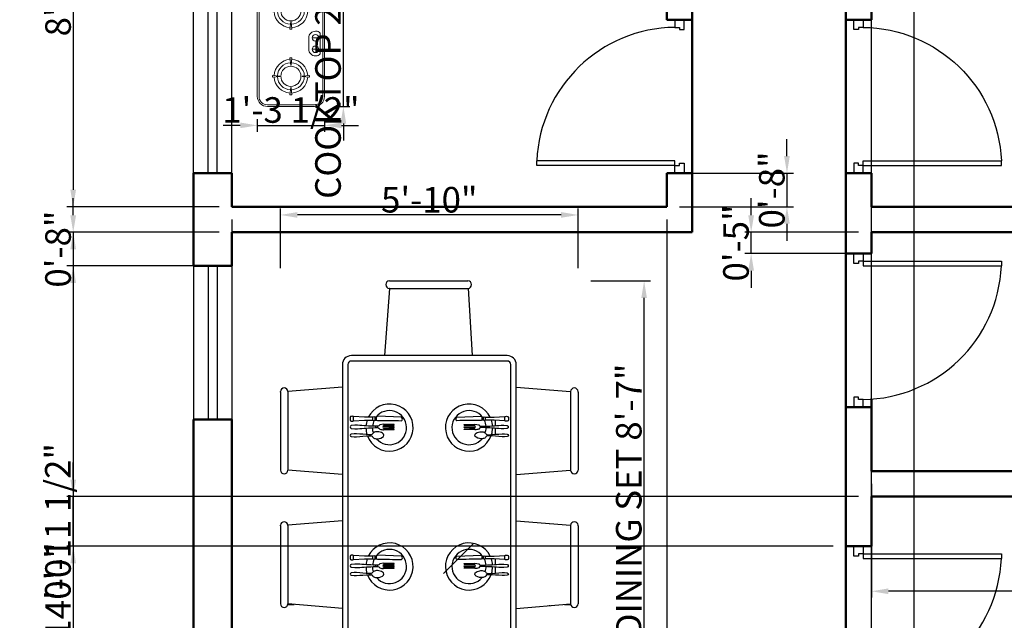
# Model space of a CAD drawing. Units: inches. Extents: x 749 to 1130, y 885 to 1490.
# Tile 3 of 5: x 749 to 980, y 1204 to 1345. Entities that reach past the tile are written whole.
import ezdxf

# ---------------------------------------------------------------- set-up
doc = ezdxf.new("R2010")
doc.units = ezdxf.units.IN
doc.header["$MEASUREMENT"] = 0
doc.layers.add('a patt', color=33, linetype='Continuous')
for name, color, linetype, lineweight in [('A-ANNO-DIMS', 2, 'Continuous', 18), ('A-DOOR', 2, 'Continuous', 25), ('A-EQPM', 8, 'Continuous', 20), ('A-FURN', 9, 'Continuous', 18), ('WALL', 7, 'Continuous', 50), ('WINDOW', 2, 'Continuous', 25)]:
    doc.layers.add(name, color=color, linetype=linetype, lineweight=lineweight)
doc.styles.get("Standard").update_dxf_attribs({"font": 'arial.ttf'})
doc.dimstyles.new('yqi0', dxfattribs={"dimscale": 0, "dimtxt": 6, "dimasz": 4, "dimexe": 1.5, "dimexo": 3, "dimgap": 0.5, "dimtad": 1, "dimdsep": 46, "dimlunit": 4, "dimtxsty": 'Standard', "dimcen": 0, "dimclrd": 256, "dimclre": 256, "dimclrt": 7, "dimadec": 1, "dimazin": 2, "dimtfac": 1, "dimtix": 1, "dimtmove": 2, "dimatfit": 2, "dimfxl": 1, "dimtolj": 1, "dimtzin": 0, "dimarcsym": 0})

# ---------------------------------------------------------------- blocks, each defined once
blk = doc.blocks.new('WD_WIN4')
for p, q in [((-0.5, 0.5), (0.5, 0.5)), ((-0.5, 0.12), (0.5, 0.12)), ((-0.5, -0.12), (0.5, -0.12)), ((-0.5, -0.5), (0.5, -0.5))]:
    blk.add_line(p, q)
blk = doc.blocks.new('DR_D01')
for p, q in [((-0.45, 0.93), (-0.42, 0.93)), ((-0.45, 0.03), (-0.45, 0.93)), ((-0.42, 0.03), (-0.42, 0.93)), ((-0.5, 0.03), (-0.42, 0.03)), ((-0.5, 0.03), (-0.5, -0.03)), ((-0.45, 0.03), (-0.45, 0)), ((-0.45, 0), (-0.435, 0)), ((-0.435, 0), (-0.435, -0.03)), ((0.435, 0), (0.435, -0.03)), ((0.45, 0), (0.435, 0)), ((0.45, 0.03), (0.45, 0)), ((0.5, 0.03), (0.45, 0.03)), ((0.5, -0.03), (0.5, 0.03)), ((-0.435, -0.03), (-0.5, -0.03)), ((0.435, -0.03), (0.5, -0.03))]:
    blk.add_line(p, q)
blk.add_arc((-0.4602, 0.0206), 0.9103, 0.59152, 87.46644)
blk = doc.blocks.new('yq_cooker_01')
for p, q in [((426.3, 34.3), (465.5, 34.3)), ((426.3, -34.3), (465.5, -34.3))]:
    blk.add_line(p, q)
for points in [[(440, -375), (160, -375, -0.414214), (100, -315), (100, 315, -0.414214), (160, 375), (440, 375, -0.414214), (500, 315), (500, -315, -0.414214)], [(440, -365), (160, -365, -0.414214), (110, -315), (110, 315, -0.414214), (160, 365), (440, 365, -0.414214), (490, 315), (490, -315, -0.414214)]]:
    blk.add_lwpolyline(points, format="xyb", close=True)
for points in [[(300.8, 261.3), (305.4, 305), (294.6, 305), (299.2, 261.3)], [(233.7, 195.8), (190, 200.4), (190, 189.6), (233.7, 194.2)], [(366.3, 194.2), (410, 189.6), (410, 200.4), (366.3, 195.8)], [(299.2, 128.7), (294.6, 85), (305.4, 85), (300.8, 128.7)], [(299.2, -128.7), (294.6, -85), (305.4, -85), (300.8, -128.7)], [(233.7, -195.8), (190, -200.4), (190, -189.6), (233.7, -194.2)], [(366.3, -194.2), (410, -189.6), (410, -200.4), (366.3, -195.8)], [(300.8, -261.3), (305.4, -305), (294.6, -305), (299.2, -261.3)]]:
    blk.add_lwpolyline(points, close=True)
blk.add_lwpolyline([(406.7, -34.3, 0.414214), (445.9, -73.5), (455.5, -73.5, 0.414214), (475.1, -53.9), (475.1, 53.9, 0.414214), (455.5, 73.5), (445.9, 73.5, 0.414214), (406.7, 34.3), (406.7, -34.3)], format="xyb")
for centre, radius in [((300, 195), 60), ((445.9, 34.3), 19.6), ((445.9, -34.3), 19.6), ((300, -195), 60)]:
    blk.add_circle(centre, radius)
for centre, radius, start, end in [((300, 195), 100, 92.4978, 177.5022), ((300, 195), 100, 2.4978, 87.5022), ((300, 195), 80, 91.59131, 178.40869), ((300, 195), 80, 1.59131, 88.40869), ((300, 195), 100, 182.4978, 267.5022), ((300, 195), 80, 181.59131, 268.40869), ((300, 195), 80, 271.59131, 358.40869), ((300, 195), 100, 272.4978, 357.5022), ((300, -195), 100, 92.4978, 177.5022), ((300, -195), 80, 91.59131, 178.40869), ((300, -195), 80, 1.59131, 88.40869), ((300, -195), 100, 2.4978, 87.5022), ((300, -195), 100, 182.4978, 267.5022), ((300, -195), 80, 181.59131, 268.40869), ((300, -195), 80, 271.59131, 358.40869), ((300, -195), 100, 272.4978, 357.5022)]:
    blk.add_arc(centre, radius, start, end)
blk = doc.blocks.new('grdfg')
at = {"layer": 'a patt'}
for p, q in [((615.1, 1349.1), (612, 1348.9)), ((1015.8, 1349), (615, 1349)), ((615, 1348.9), (615, 1349)), ((1015.8, 1349.1), (1018.9, 1348.9)), ((1307.5, 1349.1), (1304.3, 1348.9)), ((1307.4, 1348.9), (1307.4, 1349)), ((1708.1, 1349), (1307.4, 1349)), ((1708.1, 1349.1), (1711.2, 1348.9)), ((589, 1028.2), (611.9, 1309.9)), ((609.3, 1310.2), (609.3, 1278.3)), ((1018.9, 1309.9), (611.8, 1309.9)), ((1041.8, 1028.2), (1018.9, 1310)), ((1281.4, 1028.2), (1304.2, 1309.9)), ((1711.2, 1309.9), (1304.2, 1309.9)), ((1734.1, 1028.2), (1711.3, 1310)), ((605.1, 1201.3), (603.1, 1201.3)), ((1297.4, 1201.3), (1295.4, 1201.3)), ((1850.7, 1028.2), (443.9, 1028.2)), ((397.3, 981.6), (397.3, 174.8)), ((425.3, 981.6), (425.3, 174.8)), ((1850.7, 1000.2), (443.9, 1000.2)), ((841.2, 969.6), (862.7, 969.6)), ((1560.1, 969.6), (1581.7, 969.6)), ((1869.3, 174.8), (1869.3, 981.6)), ((1897.3, 174.8), (1897.3, 981.6)), ((763.3, 888.1), (769.2, 888.1)), ((763.3, 878.9), (769.2, 878.9)), ((844.8, 869.7), (859.1, 869.7)), ((1482.3, 888.1), (1488.2, 888.1)), ((1482.3, 878.9), (1488.2, 878.9)), ((1563.7, 869.7), (1578.1, 869.7)), ((812.6, 857.1), (805.6, 857.1)), ((805.6, 844.8), (812.6, 844.8)), ((844.8, 858.9), (859.1, 858.9)), ((844.8, 851.7), (859.1, 851.7)), ((1531.6, 857.1), (1524.6, 857.1)), ((1524.6, 844.8), (1531.6, 844.8)), ((1563.7, 858.9), (1578.1, 858.9)), ((1563.7, 851.7), (1578.1, 851.7)), ((10, 784.9), (10, 377.8)), ((49.2, 781.8), (49, 784.9)), ((397.3, 807.5), (49.1, 781.7)), ((49.1, 781.7), (49.1, 381)), ((1897.3, 807.5), (2245.5, 781.7)), ((2245.4, 781.8), (2245.6, 784.9)), ((2245.5, 781.7), (2245.5, 381)), ((2284.6, 784.9), (2284.6, 377.8)), ((769.7, 504.8), (923, 351.5)), ((397.3, 355.1), (48.7, 375)), ((49.2, 381.1), (49, 378)), ((49, 381), (49.1, 381)), ((1897.3, 355.1), (2245.9, 375)), ((2245.4, 381.1), (2245.6, 378)), ((2245.6, 381), (2245.5, 381)), ((805.6, 311.6), (812.6, 311.6)), ((1524.6, 311.6), (1531.6, 311.6)), ((763.3, 277.5), (769.2, 277.5)), ((763.3, 268.3), (769.2, 268.3)), ((812.6, 299.3), (805.6, 299.3)), ((844.8, 304.7), (859.1, 304.7)), ((844.8, 297.5), (859.1, 297.5)), ((844.8, 286.7), (859.1, 286.7)), ((1482.3, 277.5), (1488.2, 277.5)), ((1482.3, 268.3), (1488.2, 268.3)), ((1531.6, 299.3), (1524.6, 299.3)), ((1563.7, 304.7), (1578.1, 304.7)), ((1563.7, 297.5), (1578.1, 297.5)), ((1563.7, 286.7), (1578.1, 286.7)), ((771, 235), (802.4, 235)), ((815.8, 235), (844.3, 235)), ((1490, 235), (1521.4, 235)), ((1534.8, 235), (1563.3, 235)), ((443.9, 156.2), (1850.7, 156.2)), ((841.2, 186.8), (862.7, 186.8)), ((1560.1, 186.8), (1581.7, 186.8)), ((443.9, 128.2), (1850.7, 128.2)), ((589, 128.2), (611.9, -153.5)), ((1041.8, 128.2), (1018.9, -153.6)), ((1281.4, 128.2), (1304.2, -153.5)), ((1734.1, 128.2), (1711.3, -153.6)), ((605.1, -44.9), (603.1, -44.9)), ((1027.7, -44.9), (1025.6, -44.9)), ((609.3, -122), (609.3, -153.8)), ((1018.9, -153.5), (611.8, -153.5)), ((615.1, -192.7), (612, -192.5)), ((615, -192.5), (615, -192.6)), ((1015.8, -192.6), (615, -192.6)), ((1015.8, -192.7), (1018.9, -192.5)), ((1711.2, -153.5), (1304.2, -153.5)), ((1307.5, -192.7), (1304.3, -192.5)), ((1307.4, -192.5), (1307.4, -192.6)), ((1708.1, -192.6), (1307.4, -192.6)), ((1708.1, -192.7), (1711.2, -192.5))]:
    blk.add_line(p, q, dxfattribs=at)
for points in [[(758.7, 967), (758.7, 954.7, -0.013852), (763.3, 888.1), (763.3, 878.9, -0.321801), (757.9, 871.5, 0.220637), (748.8, 856.4, 0.151079), (755.6, 820.3, 0.601255), (776.8, 820.3, 0.098298), (784.5, 845.7, 0.173345), (779.1, 866.9, 0.127575), (772.3, 873, -0.108886), (769.2, 878.9), (769.2, 888.1, -0.013852), (773.8, 954.7), (773.8, 967), (772.3, 982, 0.903848), (760.2, 982)], [(841.2, 985.7, 0.204141), (841.2, 969.6), (844.8, 914.2), (844.8, 869.7), (843, 862.5), (844.8, 858.9), (844.8, 851.7), (843, 846.6, -0.015744), (841.2, 721.5, 0.538165), (859.1, 721.5), (864.3, 846.6), (859.1, 851.7), (859.1, 858.9), (860.9, 862.5), (859.1, 869.7), (859.1, 914.2), (862.7, 969.6, 0.204141), (862.7, 985.7), (857.3, 987.5), (846.6, 987.5)], [(1477.7, 967), (1477.7, 954.7, -0.013852), (1482.3, 888.1), (1482.3, 878.9, -0.321801), (1476.9, 871.5, 0.220637), (1467.8, 856.4, 0.151079), (1474.6, 820.3, 0.601255), (1495.8, 820.3, 0.098298), (1503.5, 845.7, 0.173345), (1498.1, 866.9, 0.127575), (1491.2, 873, -0.108886), (1488.2, 878.9), (1488.2, 888.1, -0.013852), (1492.8, 954.7), (1492.8, 967), (1491.2, 982, 0.903848), (1479.2, 982)], [(1560.1, 985.7, 0.204141), (1560.1, 969.6), (1563.7, 914.2), (1563.7, 869.7), (1561.9, 862.5), (1563.7, 858.9), (1563.7, 851.7), (1561.9, 846.6, -0.015744), (1560.1, 721.5, 0.538165), (1578.1, 721.5), (1583.3, 846.6), (1578.1, 851.7), (1578.1, 858.9), (1579.9, 862.5), (1578.1, 869.7), (1578.1, 914.2), (1581.7, 969.6, 0.204141), (1581.7, 985.7), (1576.3, 987.5), (1565.5, 987.5)], [(841.2, 170.6, -0.204141), (841.2, 186.8), (844.8, 242.1), (844.8, 286.7), (843, 293.9), (844.8, 297.5), (844.8, 304.7), (843, 309.8, 0.015744), (841.2, 434.9, -0.538165), (859.1, 434.9), (864.3, 309.8), (859.1, 304.7), (859.1, 297.5), (860.9, 293.9), (859.1, 286.7), (859.1, 242.1), (862.7, 186.8, -0.204141), (862.7, 170.6), (857.3, 168.8), (846.6, 168.8)], [(1560.1, 170.6, -0.204141), (1560.1, 186.8), (1563.7, 242.1), (1563.7, 286.7), (1561.9, 293.9), (1563.7, 297.5), (1563.7, 304.7), (1561.9, 309.8, 0.015744), (1560.1, 434.9, -0.538165), (1578.1, 434.9), (1583.3, 309.8), (1578.1, 304.7), (1578.1, 297.5), (1579.9, 293.9), (1578.1, 286.7), (1578.1, 242.1), (1581.7, 186.8, -0.204141), (1581.7, 170.6), (1576.3, 168.8), (1565.5, 168.8)], [(758.7, 189.4), (758.7, 201.7, 0.013852), (763.3, 268.3), (763.3, 277.5, 0.321801), (757.9, 284.9, -0.220637), (748.8, 300, -0.151079), (755.6, 336.1, -0.601255), (776.8, 336.1, -0.098298), (784.5, 310.7, -0.173345), (779.1, 289.5, -0.127575), (772.3, 283.4, 0.108886), (769.2, 277.5), (769.2, 268.3, 0.013852), (773.8, 201.7), (773.8, 189.4), (772.3, 174.3, -0.903848), (760.2, 174.3)], [(1477.7, 189.4), (1477.7, 201.7, 0.013852), (1482.3, 268.3), (1482.3, 277.5, 0.321801), (1476.9, 284.9, -0.220637), (1467.8, 300, -0.151079), (1474.6, 336.1, -0.601255), (1495.8, 336.1, -0.098298), (1503.5, 310.7, -0.173345), (1498.1, 289.5, -0.127575), (1491.2, 283.4, 0.108886), (1488.2, 277.5), (1488.2, 268.3, 0.013852), (1492.8, 201.7), (1492.8, 189.4), (1491.2, 174.3, -0.903848), (1479.2, 174.3)]]:
    blk.add_lwpolyline(points, format="xyb", close=True, dxfattribs=at)
for points in [[(802, 981.9), (800.2, 964.2), (800.2, 950, -0.012883), (805.6, 857.1), (805.6, 844.8, -0.236068), (798.4, 834, 0.098033), (794.8, 814.4), (796.6, 759.1), (798.4, 759.1), (800.2, 814.4), (802, 814.4), (803.8, 759.1), (805.6, 759.1), (807.4, 816.2), (809.2, 818), (810.8, 816.2), (812.6, 759.1), (814.4, 759.1), (816.2, 814.4), (818, 814.4), (819.8, 759.1), (821.6, 759.1), (823.4, 814.4), (819.8, 834, -0.236068), (812.6, 844.8), (812.6, 857.1, -0.012883), (818, 950), (818, 964.2), (816.2, 981.9, 0.761905), (802, 981.9, 0.027392)], [(1521, 981.9), (1519.2, 964.2), (1519.2, 950, -0.012883), (1524.6, 857.1), (1524.6, 844.8, -0.236068), (1517.4, 834, 0.098033), (1513.8, 814.4), (1515.6, 759.1), (1517.4, 759.1), (1519.2, 814.4), (1521, 814.4), (1522.8, 759.1), (1524.6, 759.1), (1526.4, 816.2), (1528.2, 818), (1529.8, 816.2), (1531.6, 759.1), (1533.4, 759.1), (1535.2, 814.4), (1537, 814.4), (1538.8, 759.1), (1540.6, 759.1), (1542.4, 814.4), (1538.8, 834, -0.236068), (1531.6, 844.8), (1531.6, 857.1, -0.012883), (1537, 950), (1537, 964.2), (1535.2, 981.9, 0.761905), (1521, 981.9, 0.027392)], [(802, 174.5), (800.2, 192.2), (800.2, 206.4, 0.012883), (805.6, 299.3), (805.6, 311.6, 0.236068), (798.4, 322.4, -0.098033), (794.8, 342), (796.6, 397.3), (798.4, 397.3), (800.2, 342), (802, 342), (803.8, 397.3), (805.6, 397.3), (807.4, 340.2), (809.2, 338.4), (810.8, 340.2), (812.6, 397.3), (814.4, 397.3), (816.2, 342), (818, 342), (819.8, 397.3), (821.6, 397.3), (823.4, 342), (819.8, 322.4, 0.236068), (812.6, 311.6), (812.6, 299.3, 0.012883), (818, 206.4), (818, 192.2), (816.2, 174.5, -0.761905), (802, 174.5, -0.027392)], [(1521, 174.5), (1519.2, 192.2), (1519.2, 206.4, 0.012883), (1524.6, 299.3), (1524.6, 311.6, 0.236068), (1517.4, 322.4, -0.098033), (1513.8, 342), (1515.6, 397.3), (1517.4, 397.3), (1519.2, 342), (1521, 342), (1522.8, 397.3), (1524.6, 397.3), (1526.4, 340.2), (1528.2, 338.4), (1529.8, 340.2), (1531.6, 397.3), (1533.4, 397.3), (1535.2, 342), (1537, 342), (1538.8, 397.3), (1540.6, 397.3), (1542.4, 342), (1538.8, 322.4, 0.236068), (1531.6, 311.6), (1531.6, 299.3, 0.012883), (1537, 206.4), (1537, 192.2), (1535.2, 174.5, -0.761905), (1521, 174.5, -0.027392)]]:
    blk.add_lwpolyline(points, format="xyb", dxfattribs=at)
for centre, radius, start, end in [((612.9, 1329.4), 19.5, 92.4912, 267.9051), ((1018, 1329.4), 19.5, 272.0949, 87.5088), ((1305.2, 1329.4), 19.5, 92.4912, 267.9051), ((1710.4, 1329.4), 19.5, 272.0949, 87.5088), ((443.9, 981.6), 46.6, 90, 180), ((1850.7, 981.6), 46.6, 0, 90), ((443.9, 981.6), 18.7, 90, 180), ((1850.7, 981.6), 18.7, 0, 90), ((805.7, 784), 122.1, 110.569, 64.0676), ((805.7, 784), 122.1, 91.1026, 107.1168), ((805.7, 784), 88.4, 90.4281, 108.0635), ((805.7, 784), 88.4, 64.8376, 85.191), ((805.7, 784), 122.1, 71.3681, 85.7295), ((1524.7, 784), 122.1, 110.569, 64.0676), ((1524.7, 784), 122.1, 91.1026, 107.1168), ((1524.7, 784), 88.4, 90.4281, 108.0635), ((1524.7, 784), 88.4, 64.8376, 85.191), ((1524.7, 784), 122.1, 71.3681, 85.7295), ((805.7, 784), 88.4, 130.4177, 52.8326), ((1524.7, 784), 88.4, 130.4177, 52.8326), ((29.5, 784), 19.5, 2.4912, 177.9051), ((2265.1, 784), 19.5, 2.0949, 177.5088), ((805.7, 372.4), 122.1, 295.9324, 249.431), ((805.7, 372.4), 88.4, 307.1674, 229.5823), ((1524.7, 372.4), 122.1, 295.9324, 249.431), ((1524.7, 372.4), 88.4, 307.1674, 229.5823), ((29.5, 378.8), 19.5, 182.0949, 357.5088), ((2265.1, 378.8), 19.5, 182.4912, 357.9051), ((805.7, 372.4), 122.1, 252.8832, 268.8974), ((805.7, 372.4), 88.4, 251.9365, 269.5719), ((805.7, 372.4), 88.4, 274.809, 295.1624), ((805.7, 372.4), 122.1, 274.2705, 288.6319), ((1524.7, 372.4), 122.1, 252.8832, 268.8974), ((1524.7, 372.4), 88.4, 251.9365, 269.5719), ((1524.7, 372.4), 88.4, 274.809, 295.1624), ((1524.7, 372.4), 122.1, 274.2705, 288.6319), ((443.9, 174.8), 46.6, 180, 270), ((443.9, 174.8), 18.7, 180, 270), ((1850.7, 174.8), 46.6, 270, 0), ((1850.7, 174.8), 18.7, 270, 0), ((612.9, -173), 19.5, 92.0949, 267.5088), ((1018, -173), 19.5, 272.4912, 87.9051), ((1305.2, -173), 19.5, 92.0949, 267.5088), ((1710.4, -173), 19.5, 272.4912, 87.9051)]:
    blk.add_arc(centre, radius, start, end, dxfattribs=at)
blk = doc.blocks.new('*D27')
at = {"layer": 'A-ANNO-DIMS', "lineweight": -2, "transparency": 16777216}
for p, q in [((825.23, 1358.5), (825.23, 1362.5)), ((823.8, 1354.5), (826.73, 1354.5)), ((825.23, 1324.97), (825.23, 1354.5)), ((823.8, 1324.97), (826.73, 1324.97)), ((825.23, 1320.97), (825.23, 1316.97))]:
    blk.add_line(p, q, dxfattribs=at)
at = {"layer": 'A-ANNO-DIMS', "transparency": 16777216}
for points in [[(824.56, 1358.5), (825.9, 1358.5), (825.23, 1354.5)], [(824.56, 1320.97), (825.9, 1320.97), (825.23, 1324.97)]]:
    blk.add_solid(points, dxfattribs=at)
at = {"layer": 'Defpoints', "color": 0, "transparency": 16777216}
for p in [(820.8, 1354.5), (825.23, 1354.5), (820.8, 1324.97)]:
    blk.add_point(p, dxfattribs=at)
at = {"layer": 'A-ANNO-DIMS', "color": 7, "transparency": 16777216, "insert": (821.63, 1339.73), "char_height": 6, "attachment_point": 5, "rotation": 90}
blk.add_mtext('\\A1;COOKTOP 2\'-5 1/2"', dxfattribs=at)
blk = doc.blocks.new('*D28')
at = {"layer": 'A-ANNO-DIMS', "lineweight": -2, "transparency": 16777216}
for p, q in [((805.05, 1321.97), (805.05, 1319.04)), ((820.8, 1321.97), (820.8, 1319.04)), ((801.05, 1320.54), (797.05, 1320.54)), ((805.05, 1320.54), (820.8, 1320.54)), ((824.8, 1320.54), (828.8, 1320.54))]:
    blk.add_line(p, q, dxfattribs=at)
at = {"layer": 'A-ANNO-DIMS', "transparency": 16777216}
for points in [[(801.05, 1321.21), (801.05, 1319.88), (805.05, 1320.54)], [(824.8, 1321.21), (824.8, 1319.88), (820.8, 1320.54)]]:
    blk.add_solid(points, dxfattribs=at)
at = {"layer": 'Defpoints', "color": 0, "transparency": 16777216}
for p in [(805.05, 1324.97), (820.8, 1324.97), (820.8, 1320.54)]:
    blk.add_point(p, dxfattribs=at)
at = {"layer": 'A-ANNO-DIMS', "color": 7, "transparency": 16777216, "insert": (812.93, 1324.15), "char_height": 6, "attachment_point": 5}
blk.add_mtext('\\A1;1\'-3 1/2"', dxfattribs=at)
blk = doc.blocks.new('*D29')
at = {"layer": 'A-ANNO-DIMS', "lineweight": -2, "transparency": 16777216}
for p, q in [((883.31, 1284.07), (897.27, 1284.07)), ((895.77, 1185.01), (895.77, 1280.07)), ((883.31, 1181.01), (897.27, 1181.01))]:
    blk.add_line(p, q, dxfattribs=at)
at = {"layer": 'A-ANNO-DIMS', "transparency": 16777216}
for points in [[(895.1, 1280.07), (896.43, 1280.07), (895.77, 1284.07)], [(895.1, 1185.01), (896.43, 1185.01), (895.77, 1181.01)]]:
    blk.add_solid(points, dxfattribs=at)
at = {"layer": 'Defpoints', "color": 0, "transparency": 16777216}
for p in [(880.31, 1284.07), (895.77, 1284.07), (880.31, 1181.01)]:
    blk.add_point(p, dxfattribs=at)
at = {"layer": 'A-ANNO-DIMS', "color": 7, "transparency": 16777216, "insert": (892.16, 1232.54), "char_height": 6, "attachment_point": 5, "rotation": 90}
blk.add_mtext('\\A1;DINING SET 8\'-7"', dxfattribs=at)
blk = doc.blocks.new('*D30')
at = {"layer": 'A-ANNO-DIMS', "lineweight": -2, "transparency": 16777216}
for p, q in [((810.45, 1287.07), (810.45, 1301.03)), ((880.31, 1287.07), (880.31, 1301.03)), ((876.31, 1299.53), (814.45, 1299.53))]:
    blk.add_line(p, q, dxfattribs=at)
at = {"layer": 'A-ANNO-DIMS', "transparency": 16777216}
for points in [[(814.45, 1300.2), (814.45, 1298.87), (810.45, 1299.53)], [(876.31, 1300.2), (876.31, 1298.87), (880.31, 1299.53)]]:
    blk.add_solid(points, dxfattribs=at)
at = {"layer": 'Defpoints', "color": 0, "transparency": 16777216}
for p in [(810.45, 1299.53), (810.45, 1284.07), (880.31, 1284.07)]:
    blk.add_point(p, dxfattribs=at)
at = {"layer": 'A-ANNO-DIMS', "color": 7, "transparency": 16777216, "insert": (845.38, 1303.1), "char_height": 6, "attachment_point": 5}
blk.add_mtext('\\A1;5\'-10"', dxfattribs=at)
blk = doc.blocks.new('*D33')
at = {"layer": 'A-ANNO-DIMS', "lineweight": -2, "transparency": 16777216}
for p, q in [((796.07, 1399.46), (760.37, 1399.46)), ((761.87, 1395.46), (761.87, 1305.46)), ((796.07, 1301.46), (760.37, 1301.46))]:
    blk.add_line(p, q, dxfattribs=at)
at = {"layer": 'A-ANNO-DIMS', "transparency": 16777216}
for points in [[(761.2, 1395.46), (762.54, 1395.46), (761.87, 1399.46)], [(761.2, 1305.46), (762.54, 1305.46), (761.87, 1301.46)]]:
    blk.add_solid(points, dxfattribs=at)
at = {"layer": 'Defpoints', "color": 0, "transparency": 16777216}
for p in [(799.07, 1399.46), (761.87, 1301.46), (799.07, 1301.46)]:
    blk.add_point(p, dxfattribs=at)
at = {"layer": 'A-ANNO-DIMS', "color": 7, "transparency": 16777216, "insert": (758.31, 1350.46), "char_height": 6, "attachment_point": 5, "rotation": 90}
blk.add_mtext('\\A1;8\'-2"', dxfattribs=at)
blk = doc.blocks.new('*D34')
at = {"layer": 'A-ANNO-DIMS', "lineweight": -2, "transparency": 16777216}
for p, q in [((796.07, 1295.46), (760.37, 1295.46)), ((761.87, 1291.46), (761.87, 1131.46)), ((796.07, 1127.46), (760.37, 1127.46))]:
    blk.add_line(p, q, dxfattribs=at)
at = {"layer": 'A-ANNO-DIMS', "transparency": 16777216}
for points in [[(761.2, 1291.46), (762.54, 1291.46), (761.87, 1295.46)], [(761.2, 1131.46), (762.54, 1131.46), (761.87, 1127.46)]]:
    blk.add_solid(points, dxfattribs=at)
at = {"layer": 'Defpoints', "color": 0, "transparency": 16777216}
for p in [(799.07, 1295.46), (761.87, 1127.46), (799.07, 1127.46)]:
    blk.add_point(p, dxfattribs=at)
at = {"layer": 'A-ANNO-DIMS', "color": 7, "transparency": 16777216, "insert": (758.31, 1211.46), "char_height": 6, "attachment_point": 5, "rotation": 90}
blk.add_mtext('\\A1;14\'-0"', dxfattribs=at)
blk = doc.blocks.new('*D41')
at = {"layer": 'A-ANNO-DIMS', "lineweight": -2, "transparency": 16777216}
for p, q in [((799.07, 1298.46), (799.07, 884.76)), ((901.07, 1298.46), (901.07, 884.76)), ((803.07, 886.26), (897.07, 886.26))]:
    blk.add_line(p, q, dxfattribs=at)
at = {"layer": 'A-ANNO-DIMS', "transparency": 16777216}
for points in [[(803.07, 886.93), (803.07, 885.59), (799.07, 886.26)], [(897.07, 886.93), (897.07, 885.59), (901.07, 886.26)]]:
    blk.add_solid(points, dxfattribs=at)
at = {"layer": 'Defpoints', "color": 0, "transparency": 16777216}
for p in [(799.07, 1301.46), (901.07, 1301.46), (901.07, 886.26)]:
    blk.add_point(p, dxfattribs=at)
at = {"layer": 'A-ANNO-DIMS', "color": 7, "transparency": 16777216, "insert": (850.07, 889.82), "char_height": 6, "attachment_point": 5}
blk.add_mtext('\\A1;8\'-6"', dxfattribs=at)
blk = doc.blocks.new('*D47')
at = {"layer": 'A-ANNO-DIMS', "lineweight": -2, "transparency": 16777216}
for p, q in [((945.07, 1482.66), (941.07, 1482.66)), ((949.07, 1087.46), (949.07, 1484.16)), ((949.07, 1482.66), (959.07, 1482.66)), ((959.07, 1087.46), (959.07, 1484.16)), ((963.07, 1482.66), (967.07, 1482.66))]:
    blk.add_line(p, q, dxfattribs=at)
at = {"layer": 'A-ANNO-DIMS', "transparency": 16777216}
for points in [[(945.07, 1483.33), (945.07, 1481.99), (949.07, 1482.66)], [(963.07, 1483.33), (963.07, 1481.99), (959.07, 1482.66)]]:
    blk.add_solid(points, dxfattribs=at)
at = {"layer": 'Defpoints', "color": 0, "transparency": 16777216}
for p in [(959.07, 1482.66), (949.07, 1084.46), (959.07, 1084.46)]:
    blk.add_point(p, dxfattribs=at)
at = {"layer": 'A-ANNO-DIMS', "color": 7, "transparency": 16777216, "insert": (954.07, 1486.22), "char_height": 6, "attachment_point": 5}
blk.add_mtext('\\A1;0\'-10"', dxfattribs=at)
blk = doc.blocks.new('*D51')
at = {"layer": 'A-ANNO-DIMS', "lineweight": -2, "transparency": 16777216}
for p, q in [((949.07, 1236.46), (949.07, 1209.76)), ((1036.07, 1236.46), (1036.07, 1209.76)), ((1032.07, 1211.26), (953.07, 1211.26))]:
    blk.add_line(p, q, dxfattribs=at)
at = {"layer": 'A-ANNO-DIMS', "transparency": 16777216}
for points in [[(953.07, 1211.93), (953.07, 1210.59), (949.07, 1211.26)], [(1032.07, 1211.93), (1032.07, 1210.59), (1036.07, 1211.26)]]:
    blk.add_solid(points, dxfattribs=at)
at = {"layer": 'Defpoints', "color": 0, "transparency": 16777216}
for p in [(949.07, 1239.46), (1036.07, 1239.46), (949.07, 1211.26)]:
    blk.add_point(p, dxfattribs=at)
at = {"layer": 'A-ANNO-DIMS', "color": 7, "transparency": 16777216, "insert": (992.57, 1214.83), "char_height": 6, "attachment_point": 5}
blk.add_mtext('\\A1;7\'-3"', dxfattribs=at)
blk = doc.blocks.new('*D54')
at = {"layer": 'A-ANNO-DIMS', "lineweight": -2, "transparency": 16777216}
for p, q in [((761.87, 1299.46), (761.87, 1303.46)), ((796.07, 1295.46), (760.37, 1295.46)), ((761.87, 1295.46), (761.87, 1287.59)), ((796.07, 1287.59), (760.37, 1287.59)), ((761.87, 1283.59), (761.87, 1279.59))]:
    blk.add_line(p, q, dxfattribs=at)
at = {"layer": 'A-ANNO-DIMS', "transparency": 16777216}
for points in [[(761.2, 1299.46), (762.54, 1299.46), (761.87, 1295.46)], [(761.2, 1283.59), (762.54, 1283.59), (761.87, 1287.59)]]:
    blk.add_solid(points, dxfattribs=at)
at = {"layer": 'Defpoints', "color": 0, "transparency": 16777216}
for p in [(799.07, 1295.46), (761.87, 1287.59), (799.07, 1287.59)]:
    blk.add_point(p, dxfattribs=at)
at = {"layer": 'A-ANNO-DIMS', "color": 7, "transparency": 16777216, "insert": (758.31, 1291.52), "char_height": 6, "attachment_point": 5, "rotation": 90}
blk.add_mtext('\\A1;0\'-8"', dxfattribs=at)
blk = doc.blocks.new('*D58')
at = {"layer": 'A-ANNO-DIMS', "lineweight": -2, "transparency": 16777216}
for p, q in [((929.27, 1313.33), (929.27, 1317.33)), ((904.07, 1309.33), (930.77, 1309.33)), ((929.27, 1309.33), (929.27, 1301.46)), ((904.07, 1301.46), (930.77, 1301.46)), ((929.27, 1297.46), (929.27, 1293.46))]:
    blk.add_line(p, q, dxfattribs=at)
at = {"layer": 'A-ANNO-DIMS', "transparency": 16777216}
for points in [[(928.6, 1313.33), (929.94, 1313.33), (929.27, 1309.33)], [(928.6, 1297.46), (929.94, 1297.46), (929.27, 1301.46)]]:
    blk.add_solid(points, dxfattribs=at)
at = {"layer": 'Defpoints', "color": 0, "transparency": 16777216}
for p in [(901.07, 1309.33), (901.07, 1301.46), (929.27, 1301.46)]:
    blk.add_point(p, dxfattribs=at)
at = {"layer": 'A-ANNO-DIMS', "color": 7, "transparency": 16777216, "insert": (925.71, 1305.4), "char_height": 6, "attachment_point": 5, "rotation": 90}
blk.add_mtext('\\A1;0\'-8"', dxfattribs=at)
blk = doc.blocks.new('*D59')
at = {"layer": 'A-ANNO-DIMS', "lineweight": -2, "transparency": 16777216}
for p, q in [((761.87, 1237.46), (761.87, 1241.46)), ((946.07, 1233.46), (760.37, 1233.46)), ((761.87, 1221.83), (761.87, 1233.46)), ((940.07, 1221.83), (760.37, 1221.83)), ((761.87, 1217.83), (761.87, 1213.83))]:
    blk.add_line(p, q, dxfattribs=at)
at = {"layer": 'A-ANNO-DIMS', "transparency": 16777216}
for points in [[(761.2, 1237.46), (762.54, 1237.46), (761.87, 1233.46)], [(761.2, 1217.83), (762.54, 1217.83), (761.87, 1221.83)]]:
    blk.add_solid(points, dxfattribs=at)
at = {"layer": 'Defpoints', "color": 0, "transparency": 16777216}
for p in [(761.87, 1233.46), (949.07, 1233.46), (943.07, 1221.83)]:
    blk.add_point(p, dxfattribs=at)
at = {"layer": 'A-ANNO-DIMS', "color": 7, "transparency": 16777216, "insert": (758.27, 1227.65), "char_height": 6, "attachment_point": 5, "rotation": 90}
blk.add_mtext('\\A1;0\'-11 1/2"', dxfattribs=at)
blk = doc.blocks.new('*D60')
at = {"layer": 'A-ANNO-DIMS', "lineweight": -2, "transparency": 16777216}
for p, q in [((920.87, 1299.46), (920.87, 1303.46)), ((946.07, 1295.46), (919.37, 1295.46)), ((920.87, 1290.46), (920.87, 1295.46)), ((946.07, 1290.46), (919.37, 1290.46)), ((920.87, 1286.46), (920.87, 1282.46))]:
    blk.add_line(p, q, dxfattribs=at)
at = {"layer": 'A-ANNO-DIMS', "transparency": 16777216}
for points in [[(920.2, 1299.46), (921.54, 1299.46), (920.87, 1295.46)], [(920.2, 1286.46), (921.54, 1286.46), (920.87, 1290.46)]]:
    blk.add_solid(points, dxfattribs=at)
at = {"layer": 'Defpoints', "color": 0, "transparency": 16777216}
for p in [(920.87, 1295.46), (949.07, 1295.46), (949.07, 1290.46)]:
    blk.add_point(p, dxfattribs=at)
at = {"layer": 'A-ANNO-DIMS', "color": 7, "transparency": 16777216, "insert": (917.31, 1292.96), "char_height": 6, "attachment_point": 5, "rotation": 90}
blk.add_mtext('\\A1;0\'-5"', dxfattribs=at)

msp = doc.modelspace()

# ---------------------------------------------------------------- linework, layer by layer
at = {"layer": 'WALL'}
for p, q in [((949.07, 1345.334), (949.07, 1445.46)), ((901.07, 1345.334), (901.07, 1399.46)), ((943.07, 1309.334), (943.07, 1399.46)), ((907.07, 1345.334), (907.07, 1351.46)), ((901.07, 1345.334), (907.07, 1345.334)), ((907.07, 1295.46), (907.07, 1345.334)), ((943.07, 1345.334), (943.07, 1345.46)), ((949.07, 1345.334), (943.07, 1345.334)), ((799.07, 1309.334), (790.07, 1309.334)), ((790.07, 1287.586), (790.07, 1309.334)), ((799.07, 1301.46), (799.07, 1309.334)), ((901.07, 1301.46), (901.07, 1309.334)), ((901.07, 1309.334), (907.07, 1309.334)), ((949.07, 1309.334), (943.07, 1309.334)), ((943.07, 1301.46), (943.07, 1309.334)), ((949.07, 1301.46), (949.07, 1309.334)), ((799.07, 1301.46), (901.07, 1301.46)), ((943.07, 1290.46), (943.07, 1301.46)), ((949.07, 1301.46), (1073.196, 1301.46)), ((799.07, 1295.46), (907.07, 1295.46)), ((799.07, 1287.586), (799.07, 1295.46)), ((949.07, 1295.46), (1036.07, 1295.46)), ((949.07, 1295.46), (949.07, 1290.46)), ((949.07, 1290.46), (943.07, 1290.46)), ((943.07, 1221.834), (943.07, 1290.46)), ((799.07, 1287.586), (790.07, 1287.586)), ((949.07, 1256.337), (949.07, 1239.46)), ((943.07, 1254.46), (949.07, 1254.46)), ((790.07, 1171.334), (790.07, 1251.586)), ((799.07, 1251.586), (790.07, 1251.586)), ((799.07, 1171.334), (799.07, 1251.586)), ((949.07, 1239.46), (1036.07, 1239.46)), ((949.07, 1233.46), (1081.07, 1233.46)), ((949.07, 1233.46), (949.07, 1221.834)), ((943.07, 1171.334), (943.07, 1221.834)), ((943.07, 1221.834), (949.07, 1221.834))]:
    msp.add_line(p, q, dxfattribs=at)

# ---------------------------------------------------------------- block references
at = {"layer": 'A-DOOR', "zscale": 36}
for p, xscale, yscale, rotation in [((904.07, 1327.334), 36, 36, 90), ((946.07, 1327.334), 36, -36, 90), ((946.07, 1272.46), 36, 36, 269.9999999999998), ((946.07, 1203.834), -36, -36, 90.00000000000017)]:
    msp.add_blockref('DR_D01', p, dxfattribs=dict(at, xscale=xscale, yscale=yscale, rotation=rotation))
at = {"layer": 'A-EQPM', "xscale": 0.0393700787401575, "yscale": 0.0393700787401575, "zscale": 0.0393700787401575}
msp.add_blockref('yq_cooker_01', (801.117, 1339.735), dxfattribs=at)
at = {"layer": 'A-FURN', "xscale": 0.0453086432222982, "yscale": 0.0453086432222982, "zscale": 0.0453086432222982, "rotation": 90}
msp.add_blockref('grdfg', (871.578, 1180.561), dxfattribs=at)
at = {"layer": 'WINDOW'}
for p, xscale, yscale, zscale, rotation in [((794.57, 1333.334), 48, 8.999999999998522, 48, 89.99999999999973), ((794.57, 1269.586), 36, 8.999999999998863, 36, 269.9999999999998)]:
    msp.add_blockref('WD_WIN4', p, dxfattribs=dict(at, xscale=xscale, yscale=yscale, zscale=zscale, rotation=rotation))

# ---------------------------------------------------------------- dimensions: what is measured, and where the dimension line sits
at = {"layer": 'A-ANNO-DIMS'}
for base, p1, p2, picture, middle in [((959.07, 1482.66), (949.07, 1084.46), (959.07, 1084.46), '*D47', (954.07, 1486.224)), ((820.802, 1320.542), (805.054, 1324.971), (820.802, 1324.971), '*D28', (812.928, 1324.146)), ((901.07, 886.26), (799.07, 1301.46), (901.07, 1301.46), '*D41', (850.07, 889.824))]:
    dim = msp.add_linear_dim(base=base, p1=p1, p2=p2, dimstyle='yqi0', override={"dimscale": 1, "dimdec": 1, "dimzin": 1, "dimfrac": 2}, dxfattribs=at)
    dim.commit()
    dim.dimension.update_dxf_attribs({"geometry": picture, "text_midpoint": middle})
for base, p1, p2, angle, picture, middle in [((761.87, 1301.46), (799.07, 1399.46), (799.07, 1301.46), 90, '*D33', (758.306, 1350.46)), ((929.27, 1301.46), (901.07, 1309.334), (901.07, 1301.46), 270, '*D58', (925.706, 1305.397)), ((810.454, 1299.534), (880.308, 1284.074), (810.454, 1284.074), 180, '*D30', (845.381, 1303.097)), ((761.87, 1287.586), (799.07, 1295.46), (799.07, 1287.586), 90, '*D54', (758.306, 1291.523)), ((920.87, 1295.46), (949.07, 1290.46), (949.07, 1295.46), 90, '*D60', (917.306, 1292.96)), ((761.87, 1127.46), (799.07, 1295.46), (799.07, 1127.46), 90, '*D34', (758.306, 1211.46)), ((761.87, 1233.46), (943.07, 1221.834), (949.07, 1233.46), 90, '*D59', (758.268, 1227.647)), ((949.07, 1211.26), (1036.07, 1239.46), (949.07, 1239.46), 180, '*D51', (992.57, 1214.826))]:
    dim = msp.add_linear_dim(base=base, p1=p1, p2=p2, angle=angle, dimstyle='yqi0', override={"dimscale": 1, "dimdec": 1, "dimzin": 1, "dimfrac": 2}, dxfattribs=at)
    dim.commit()
    dim.dimension.update_dxf_attribs({"geometry": picture, "text_midpoint": middle})
for base, p1, p2, text, picture, middle in [((825.231, 1354.498), (820.802, 1324.971), (820.802, 1354.498), 'COOKTOP <>', '*D27', (821.627, 1339.735)), ((895.767, 1284.074), (880.308, 1181.013), (880.308, 1284.074), 'DINING SET <>', '*D29', (892.165, 1232.544))]:
    dim = msp.add_linear_dim(base=base, p1=p1, p2=p2, angle=90, text=text, dimstyle='yqi0', override={"dimscale": 1, "dimdec": 1, "dimzin": 1, "dimfrac": 2}, dxfattribs=at)
    dim.commit()
    dim.dimension.update_dxf_attribs({"geometry": picture, "text_midpoint": middle})

doc.saveas('drawing.dxf')
